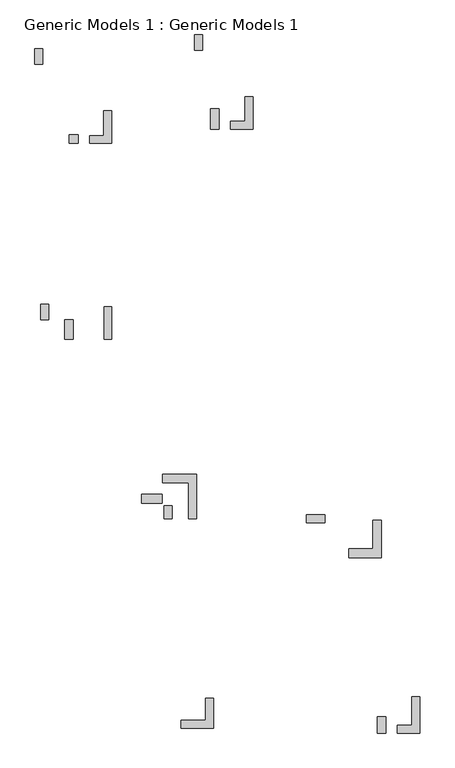
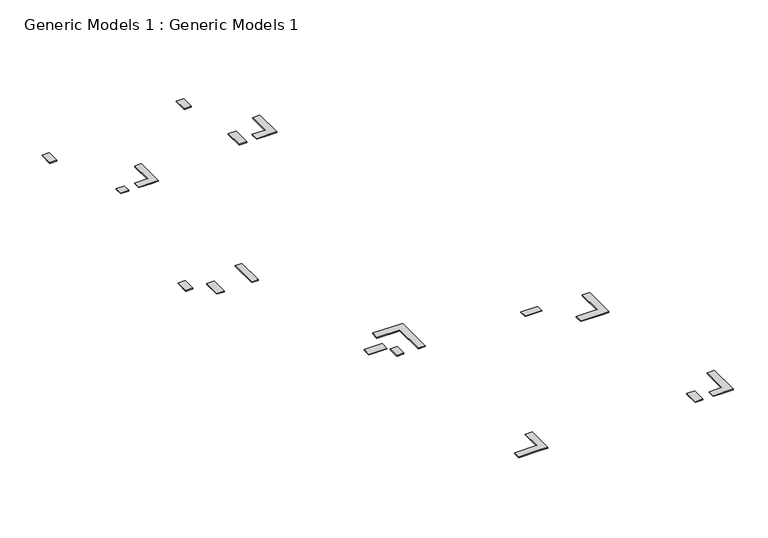
"""IFC4 building model written with IfcOpenShell, lengths in millimetres: proxy geometry, Generic Models 1 : Generic Models 1."""

from ifc_helpers import new_model, si_unit, frame, origin, place, context, project, spatial, polyline, outline, extrude, source, transform, mapped, element, save


def generic_models_1_generic_models_1_6d9a1767(model_context):
    return source(origin(), model_context, "Body", "SweptSolid", [
        extrude(outline(polyline([(-24646.9800447, 30884.0294818), (-24646.9800447, 30260.2973989), (-24646.9800447, 27580.0116713), (-25246.7640898, 27580.0116713), (-25246.7640898, 30260.2973989), (-27162.5982587, 30260.2973989), (-27162.5982587, 30884.0294818), (-24646.9800447, 30884.0294818)])), frame((0.0, 0.0, 1219.2), z_axis=(0.0, 0.0, 1.0), x_axis=(1.0, 0.0, 0.0)), (0.0, 0.0, 1.0), 76.2),
        extrude(outline(polyline([(-27219.4691188, 29383.1770746), (-27219.4691188, 28717.1999465), (-28742.7300447, 28717.1999465), (-28742.7300447, 29383.1770746), (-27219.4691188, 29383.1770746)])), frame((0.0, 0.0, 1219.2), z_axis=(0.0, 0.0, 1.0), x_axis=(1.0, 0.0, 0.0)), (0.0, 0.0, 1.0), 76.2),
        extrude(outline(polyline([(-27067.0691188, 27580.0116713), (-27067.0691188, 28530.9770746), (-26457.4691188, 28530.9770746), (-26457.4691188, 27580.0116713), (-27067.0691188, 27580.0116713)])), frame((0.0, 0.0, 1219.2), z_axis=(0.0, 0.0, 1.0), x_axis=(1.0, 0.0, 0.0)), (0.0, 0.0, 1.0), 76.2),
        extrude(outline(polyline([(-23964.2542554, 12011.8294818), (-25808.4563508, 12011.8294818), (-25808.4563508, 12603.8220475), (-23964.2542554, 12603.8220475), (-23964.2542554, 14259.8310818), (-23395.3901022, 14259.8310818), (-23395.3901022, 12011.8294818), (-23964.2542554, 12011.8294818)])), frame((0.0, 0.0, 1219.2), z_axis=(0.0, 0.0, 1.0), x_axis=(1.0, 0.0, 0.0)), (0.0, 0.0, 1.0), 76.2),
        extrude(outline(polyline([(-8645.9560644, 11663.0633156), (-9720.1419991, 11663.0633156), (-9720.1419991, 12253.3135511), (-8645.9560644, 12253.3135511), (-8645.9560644, 14375.9736639), (-8043.7419991, 14375.9736639), (-8043.7419991, 11663.0633156), (-8645.9560644, 11663.0633156)])), frame((0.0, 0.0, 1219.2), z_axis=(0.0, 0.0, 1.0), x_axis=(1.0, 0.0, 0.0)), (0.0, 0.0, 1.0), 76.2),
        extrude(outline(polyline([(-11225.1935991, 11663.0633156), (-11225.1935991, 12857.8214309), (-10583.7419991, 12857.8214309), (-10583.7419991, 11663.0633156), (-11225.1935991, 11663.0633156)])), frame((0.0, 0.0, 1219.2), z_axis=(0.0, 0.0, 1.0), x_axis=(1.0, 0.0, 0.0)), (0.0, 0.0, 1.0), 76.2),
        extrude(outline(polyline([(-15090.4456172, 27256.961205), (-16484.7370231, 27256.961205), (-16484.7370231, 27851.5253615), (-15090.4456172, 27851.5253615), (-15090.4456172, 27256.961205)])), frame((0.0, 0.0, 1219.2), z_axis=(0.0, 0.0, 1.0), x_axis=(1.0, 0.0, 0.0)), (0.0, 0.0, 1.0), 76.2),
        extrude(outline(polyline([(-11551.2933798, 24693.7122683), (-13312.2424172, 24693.7122683), (-13312.2424172, 25338.0268102), (-11551.2933798, 25338.0268102), (-11551.2933798, 27462.3122683), (-10928.8917798, 27462.3122683), (-10928.8917798, 24693.7122683), (-11551.2933798, 24693.7122683)])), frame((0.0, 0.0, 1219.2), z_axis=(0.0, 0.0, 1.0), x_axis=(1.0, 0.0, 0.0)), (0.0, 0.0, 1.0), 76.2),
        extrude(outline(polyline([(-21056.0826048, 56461.4250546), (-22122.2772109, 56461.4250546), (-22122.2772109, 57065.2166527), (-21056.0826048, 57065.2166527), (-21056.0826048, 58901.4698597), (-20445.8772109, 58901.4698597), (-20445.8772109, 56461.4250546), (-21056.0826048, 56461.4250546)])), frame((0.0, 0.0, 1219.2), z_axis=(0.0, 0.0, 1.0), x_axis=(1.0, 0.0, 0.0)), (0.0, 0.0, 1.0), 76.2),
        extrude(outline(polyline([(-23595.4772109, 56461.4250546), (-23595.4772109, 57998.4518798), (-22960.4772109, 57998.4518798), (-22960.4772109, 56461.4250546), (-23595.4772109, 56461.4250546)])), frame((0.0, 0.0, 1219.2), z_axis=(0.0, 0.0, 1.0), x_axis=(1.0, 0.0, 0.0)), (0.0, 0.0, 1.0), 76.2),
        extrude(outline(polyline([(-24801.2202841, 63481.8982557), (-24192.4144411, 63481.8982557), (-24192.4144411, 62355.8698597), (-24801.2202841, 62355.8698597), (-24801.2202841, 63481.8982557)])), frame((0.0, 0.0, 1219.2), z_axis=(0.0, 0.0, 1.0), x_axis=(1.0, 0.0, 0.0)), (0.0, 0.0, 1.0), 76.2),
        extrude(outline(polyline([(-36060.5448409, 62442.0222557), (-36060.5448409, 61310.2998557), (-36657.2998709, 61310.2998557), (-36657.2998709, 62442.0222557), (-36060.5448409, 62442.0222557)])), frame((0.0, 0.0, 1219.2), z_axis=(0.0, 0.0, 1.0), x_axis=(1.0, 0.0, 0.0)), (0.0, 0.0, 1.0), 76.2),
        extrude(outline(polyline([(-33457.6027063, 56063.072), (-33457.6027063, 55424.4170169), (-34126.2679937, 55424.4170169), (-34126.2679937, 56063.072), (-33457.6027063, 56063.072)])), frame((0.0, 0.0, 1219.2), z_axis=(0.0, 0.0, 1.0), x_axis=(1.0, 0.0, 0.0)), (0.0, 0.0, 1.0), 76.2),
        extrude(outline(polyline([(-31530.5697105, 57855.8998557), (-30972.3442282, 57855.8998557), (-30972.3442282, 55424.4170169), (-31530.5697105, 55424.4170169), (-32602.2679937, 55424.4170169), (-32602.2679937, 56003.7178652), (-31530.5697105, 56003.7178652), (-31530.5697105, 57855.8998557)])), frame((0.0, 0.0, 1219.2), z_axis=(0.0, 0.0, 1.0), x_axis=(1.0, 0.0, 0.0)), (0.0, 0.0, 1.0), 76.2),
        extrude(outline(polyline([(-31528.8653103, 40908.6978471), (-31528.8653103, 43308.0498557), (-30972.3442282, 43308.0498557), (-30972.3442282, 40908.6978471), (-31528.8653103, 40908.6978471)])), frame((0.0, 0.0, 1219.2), z_axis=(0.0, 0.0, 1.0), x_axis=(1.0, 0.0, 0.0)), (0.0, 0.0, 1.0), 76.2),
        extrude(outline(polyline([(-33821.7634644, 42343.7978471), (-33821.7634644, 40908.6978471), (-34440.3839022, 40908.6978471), (-34440.3839022, 42343.7978471), (-33821.7634644, 42343.7978471)])), frame((0.0, 0.0, 1219.2), z_axis=(0.0, 0.0, 1.0), x_axis=(1.0, 0.0, 0.0)), (0.0, 0.0, 1.0), 76.2),
        extrude(outline(polyline([(-35620.6781634, 43479.4998557), (-35620.6781634, 42343.7978471), (-36205.5823022, 42343.7978471), (-36205.5823022, 43479.4998557), (-35620.6781634, 43479.4998557)])), frame((0.0, 0.0, 1219.2), z_axis=(0.0, 0.0, 1.0), x_axis=(1.0, 0.0, 0.0)), (0.0, 0.0, 1.0), 76.2),
    ])


if __name__ == "__main__":
    model = new_model("IFC4")
    model_context = context("Model", 3, world=origin())
    ifc_project = project(units=[si_unit("LENGTHUNIT", "METRE", prefix="MILLI")], contexts=[model_context])
    site = spatial("IfcSite", under=ifc_project)
    building = spatial("IfcBuilding", under=site)
    placement = place(None, origin())
    generic_models_1_generic_models_1_shape = generic_models_1_generic_models_1_6d9a1767(model_context)
    element("IfcBuildingElementProxy", 1, Name="Generic Models 1 : Generic Models 1", ObjectType="Generic Models 1 : Generic Models 1", at=placement, inside=building, context=model_context, shape_type="MappedRepresentation", body=[
        mapped(generic_models_1_generic_models_1_shape, transform((0.0, 0.0, 0.0), x_axis=(1.0, 0.0, 0.0), y_axis=(0.0, 1.0, 0.0), z_axis=(0.0, 0.0, 1.0))),
    ])
    save(model, "model.ifc")

# Revit data of these elements
# Element 1 (IfcBuildingElementProxy, "Generic Models 1 : Generic Models 1")
#   Materials on its faces: "OUTDOOR FLOORING"
# Materials
#   "OUTDOOR FLOORING": class "Generic", colour RGB 120 120 120, transparency 0, Cost = 0
